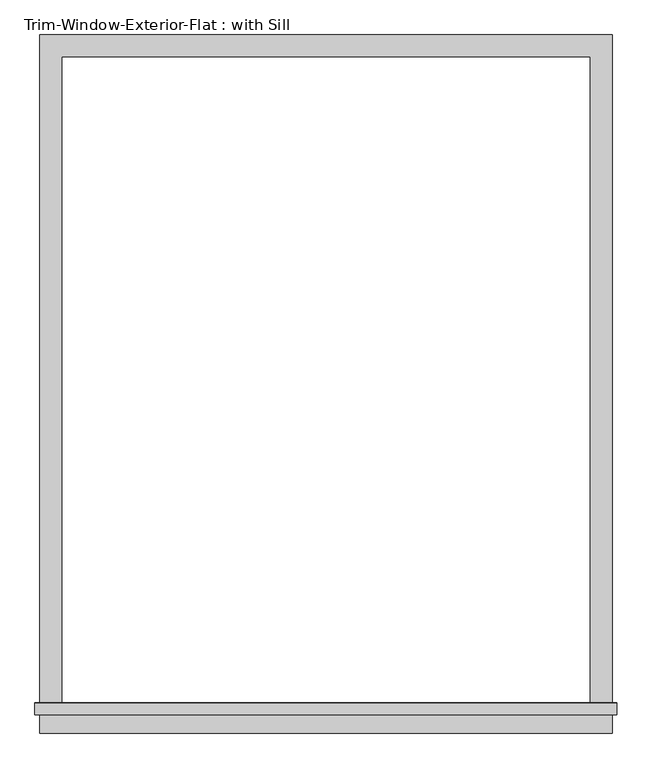
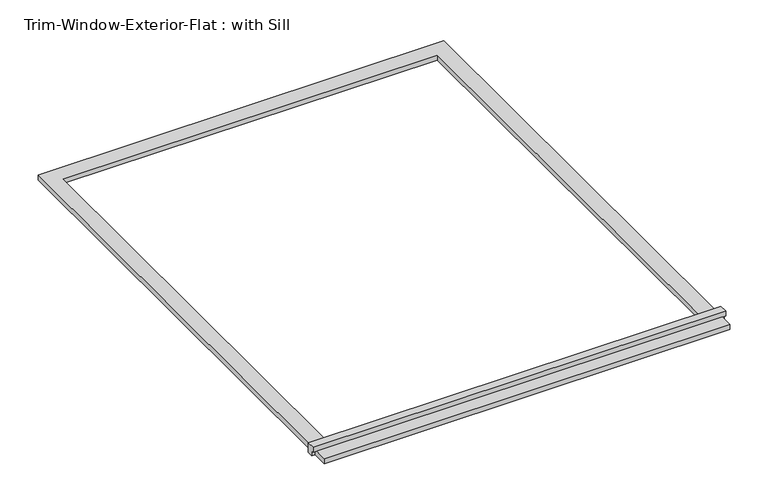
"""IFC4 building model written with IfcOpenShell, lengths in millimetres: proxy geometry, Trim-Window-Exterior-Flat : with Sill."""

from ifc_helpers import new_model, si_unit, frame, origin, origin_with_axes, place, context, project, spatial, polyline, outline, extrude, source, transform, mapped, element, save


def trim_window_exterior_flat_with_sill_f3cea81b(model_context):
    return source(origin(), model_context, "Body", "SweptSolid", [
        extrude(outline(polyline([(742.95, -1698.5823709), (742.95, -1755.7323709), (-742.95, -1755.7323709), (-742.95, -1698.5823709), (742.95, -1698.5823709)])), origin_with_axes(), (0.0, 0.0, 1.0), 19.05),
        extrude(outline(polyline([(-1708.15, 38.1), (-1678.8580645, 38.1), (-1676.4, 19.05), (-1676.4, 0.0), (-1698.5823709, 0.0), (-1698.5823709, 19.05), (-1708.15, 19.05), (-1708.15, 38.1)])), frame((-755.65, 0.0, 0.0), z_axis=(1.0, 0.0, 0.0), x_axis=(0.0, 1.0, 0.0)), (0.0, 0.0, 1.0), 1511.3),
        extrude(outline(polyline([(-742.95, 57.15), (742.95, 57.15), (742.95, -1676.4), (685.8, -1676.4), (685.8, 0.0), (-685.8, 0.0), (-685.8, -1676.4), (-742.95, -1676.4), (-742.95, 57.15)])), origin_with_axes(), (0.0, 0.0, 1.0), 19.05),
    ])


if __name__ == "__main__":
    model = new_model("IFC4")
    model_context = context("Model", 3, world=origin())
    ifc_project = project(units=[si_unit("LENGTHUNIT", "METRE", prefix="MILLI")], contexts=[model_context])
    site = spatial("IfcSite", under=ifc_project)
    building = spatial("IfcBuilding", under=site)
    placement = place(None, origin())
    trim_window_exterior_flat_with_sill_shape = trim_window_exterior_flat_with_sill_f3cea81b(model_context)
    element("IfcBuildingElementProxy", 1, Name="Trim-Window-Exterior-Flat : with Sill", ObjectType="Trim-Window-Exterior-Flat : with Sill", at=placement, inside=building, context=model_context, shape_type="MappedRepresentation", body=[
        mapped(trim_window_exterior_flat_with_sill_shape, transform((0.0, 0.0, 0.0), x_axis=(1.0, 0.0, 0.0), y_axis=(0.0, 1.0, 0.0), z_axis=(0.0, 0.0, 1.0))),
    ])
    save(model, "model.ifc")

# Revit data of these elements
# Type "Trim-Window-Exterior-Flat : with Sill"
#   Trim Width = 0' - 2 1/4"
#   Trim Thickness_Picture Frame = 0' - 1 1/4"
#   Trim Thickness_with Sill = 0' - 0 3/4"
#   Sill Thickness = 0' - 1 1/4"
#   Opening Width [instance default] = 2' - 0"
#   Opening Height [instance default] = 3' - 0"
#   Default Elevation = 4' - 0"
#   Sill = yes
#   Picture Frame = no
#   Trim Material [instance default] = none
# Element 1 (IfcBuildingElementProxy, "Trim-Window-Exterior-Flat : with Sill")
#   Opening Width = 4' - 6"
#   Opening Height = 5' - 6"
#   Trim Material = Clad - White
#   Materials on its faces: "Clad - White"
# Materials
#   "Clad - White": class "Wood", colour RGB 242 242 238, transparency 0, Cost = 0
